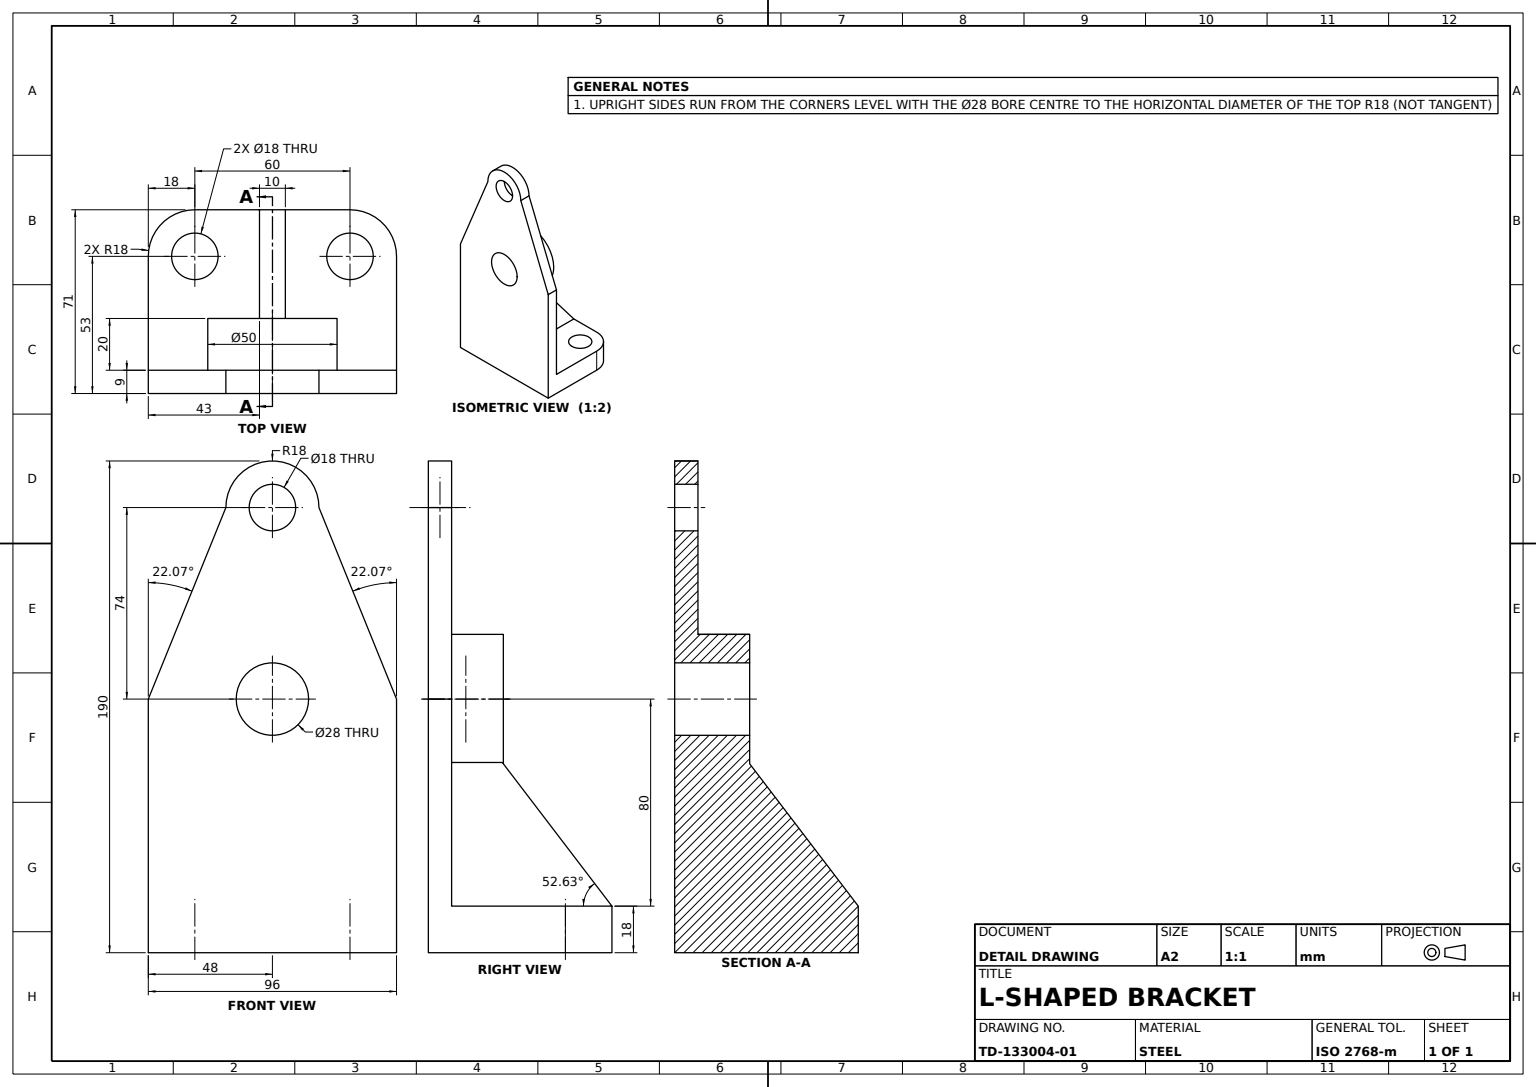
from build123d import *

# Parameters (mm, degrees)
BASE_PLATE_DEPTH          = 18
UPRIGHT_PLATE_DEPTH       = 9
UPRIGHT_TOP_HOLE_SKETCH_R = 9
UPRIGHT_TOP_HOLE_18_DEPTH = 9
HUB_BOSS_SKETCH_R         = 25
HUB_BOSS_DEPTH            = 20
HUB_BORE_SKETCH_R         = 14
HUB_BORE_28_DEPTH         = 217.979261682
BASE_HOLE_SKETCH_R        = 9
BASE_HOLE_18_DEPTH        = 225.403654159
SUPPORT_RIB_REACH         = 210.435
SUPPORT_RIB_SKETCH_WALL_W = 488.071885176
SUPPORT_RIB_SKETCH_WALL_H = 10


with BuildPart() as part:
    # Base Plate Sketch → Base Plate (new body)
    with BuildSketch(Plane(origin=(0, 0, 0), x_dir=(1, 0, 0), z_dir=(0, 1, 0))):
        with BuildLine():
            Line((0, 0), (0, 53))
            ThreePointArc((0, 53), (5.272077939, 65.727922061), (18, 71))
            Line((18, 71), (78, 71))
            ThreePointArc((78, 71), (90.727922061, 65.727922061), (96, 53))
            Line((96, 53), (96, 0))
            Line((96, 0), (0, 0))
        make_face()
    extrude(amount=BASE_PLATE_DEPTH)

    # Upright Plate Sketch → Upright Plate (add)
    with BuildSketch(Plane.XY):
        with BuildLine():
            Line((0, 98), (0, 18))
            Line((0, 18), (96, 18))
            Line((96, 18), (96, 98))
            Line((96, 98), (66, 172))
            ThreePointArc((66, 172), (48, 190), (30, 172))
            Line((30, 172), (0, 98))
        make_face()
    extrude(amount=-UPRIGHT_PLATE_DEPTH)

    # Upright Top Hole Sketch → Upright Top Hole Ø18 (cut)
    with BuildSketch(Plane(origin=(0, 0, -9), x_dir=(-1, 0, 0), z_dir=(0, 0, -1))):
        with Locations((-48, 172)):
            Circle(UPRIGHT_TOP_HOLE_SKETCH_R)
    extrude(amount=-UPRIGHT_TOP_HOLE_18_DEPTH, mode=Mode.SUBTRACT)

    # Hub Boss Sketch → Hub Boss (add)
    with BuildSketch(Plane(origin=(0, 0, -9), x_dir=(-1, 0, 0), z_dir=(0, 0, -1))):
        with Locations(Location((-48, 98, 0), (0, 0, 180))):
            Circle(HUB_BOSS_SKETCH_R)
    extrude(amount=HUB_BOSS_DEPTH)

    # Hub Bore Sketch → Hub Bore Ø28 (cut, through all)
    with BuildSketch(Plane(origin=(0, 0, -29), x_dir=(-1, 0, 0), z_dir=(0, 0, -1))):
        with Locations((-48, 98)):
            Circle(HUB_BORE_SKETCH_R)
    extrude(amount=-HUB_BORE_28_DEPTH, mode=Mode.SUBTRACT)

    # Base Hole Sketch → Base Hole Ø18 (cut, through all)
    with BuildSketch(Plane.XZ):
        with Locations(Location((18, -53, 0), (0, 0, 270))):
            Circle(BASE_HOLE_SKETCH_R)
        with Locations(Location((78, -53, 0), (0, 0, 270))):
            Circle(BASE_HOLE_SKETCH_R)
    extrude(amount=-BASE_HOLE_18_DEPTH, mode=Mode.SUBTRACT)

    # Support Rib Sketch wall → Support Rib (add, up to next)
    with BuildSketch(Plane(origin=(48, 45.5, -50), x_dir=(0, -0.794767813927, -0.606913603362), z_dir=(0, 0.606913603362, -0.794767813927)), mode=Mode.PRIVATE) as support_rib_sk1:
        Rectangle(SUPPORT_RIB_SKETCH_WALL_W, SUPPORT_RIB_SKETCH_WALL_H)
    support_rib_tool1 = extrude(support_rib_sk1.sketch, amount=-SUPPORT_RIB_REACH, mode=Mode.PRIVATE) - part.part
    add(support_rib_tool1.solids().sort_by_distance((48, 45.5, -50))[0])


solid = part.part
